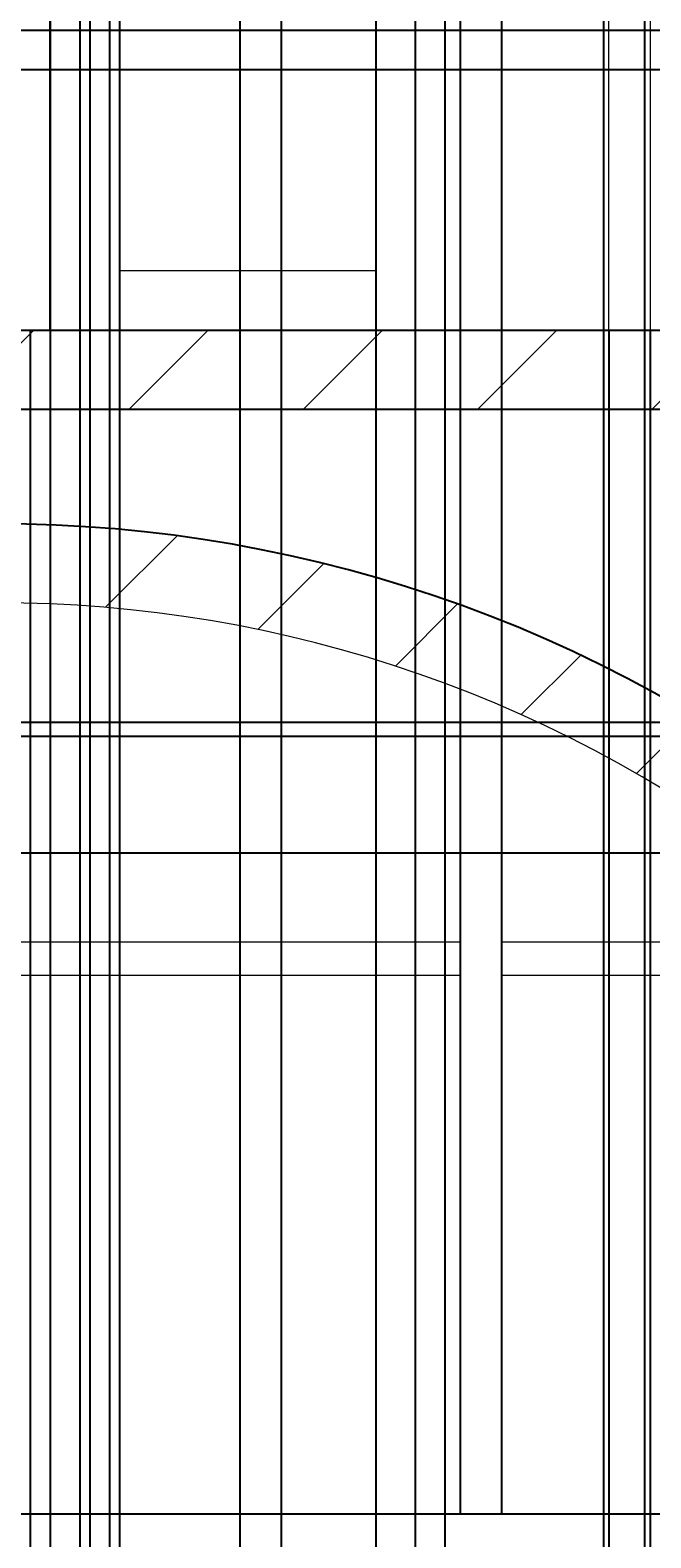
# Model space of a CAD drawing. Units: inches. Extents: x -14 to 375, y -86 to 549.
# Tile 4 of 12: x 227 to 290, y 4 to 156. Entities that reach past the tile are written whole.
import ezdxf

# ---------------------------------------------------------------- set-up
doc = ezdxf.new("R2010")
doc.units = ezdxf.units.IN
doc.header["$MEASUREMENT"] = 0
for name, color, linetype, lineweight in [('A-ANNO-DIMS', 2, 'Continuous', 18), ('A-DOOR', 3, 'Continuous', 18), ('A-ELEV', 7, 'Continuous', 25), ('A-ELEV-PATT', 8, 'Continuous', 13), ('A-GLAZ', 4, 'Continuous', 18)]:
    doc.layers.add(name, color=color, linetype=linetype, lineweight=lineweight)
doc.styles.get("Standard").update_dxf_attribs({"font": 'arial.ttf'})
doc.dimstyles.get("Standard").update_dxf_attribs({"dimtxt": 0.18, "dimasz": 0.18, "dimexe": 0.18, "dimexo": 0.0625, "dimgap": 0.09, "dimtad": 0, "dimtih": 1, "dimtoh": 1, "dimdec": 4, "dimzin": 0, "dimdsep": 46, "dimtxsty": 'Standard', "dimcen": 0.09, "dimadec": 0, "dimazin": 0, "dimtfac": 1, "dimtdec": 4, "dimtofl": 0, "dimtmove": 0, "dimatfit": 3, "dimfxl": 1, "dimtolj": 1, "dimtzin": 0, "dimarcsym": 0})

# ---------------------------------------------------------------- blocks, each defined once
blk = doc.blocks.new('*U3')
blk.add_lwpolyline([(3.12, 0.01), (0.12, 0.01), (0.12, 84.01), (40.12, 84.01), (40.12, 0.01), (37.12, 0.01)])
for points in [[(37.12, 80.99), (37.12, 0.01), (3.12, 0.01), (3.12, 80.99)], [(33.12, 6.01), (33.12, 74.99), (7.12, 74.99), (7.12, 6.01)]]:
    blk.add_lwpolyline(points, close=True)
blk.add_circle((35.12, 42.01), 1)
blk = doc.blocks.new('*D28')
at = {"layer": 'A-ANNO-DIMS', "color": 0, "lineweight": -2, "transparency": 16777216}
for p, q in [((107.764387, 156.376775), (374.544714, 156.376775)), ((374.364714, 156.196775), (374.364714, 154.556775)), ((374.364714, 152.556775), (374.364714, 154.196775)), ((111.764387, 152.376775), (374.544714, 152.376775))]:
    blk.add_line(p, q, dxfattribs=at)
at = {"layer": 'A-ANNO-DIMS', "color": 0, "transparency": 16777216}
for points in [[(374.334714, 156.196775), (374.394714, 156.196775), (374.364714, 156.376775)], [(374.334714, 152.556775), (374.394714, 152.556775), (374.364714, 152.376775)]]:
    blk.add_solid(points, dxfattribs=at)
at = {"layer": 'Defpoints', "color": 0, "transparency": 16777216}
for p in [(107.701887, 156.376775), (374.364714, 156.376775), (111.701887, 152.376775)]:
    blk.add_point(p, dxfattribs=at)
at = {"layer": 'A-ANNO-DIMS', "color": 0, "transparency": 16777216, "insert": (374.364714, 154.376775), "char_height": 0.18, "attachment_point": 5}
blk.add_mtext('\\A1;4', dxfattribs=at)
blk = doc.blocks.new('*D29')
at = {"layer": 'A-ANNO-DIMS', "color": 0, "lineweight": -2, "transparency": 16777216}
for p, q in [((107.74, 193.48), (374.54, 193.48)), ((374.36, 193.3), (374.36, 175.11)), ((374.36, 156.56), (374.36, 174.75)), ((107.76, 156.38), (374.54, 156.38))]:
    blk.add_line(p, q, dxfattribs=at)
at = {"layer": 'A-ANNO-DIMS', "color": 0, "transparency": 16777216}
for points in [[(374.33, 193.3), (374.39, 193.3), (374.36, 193.48)], [(374.33, 156.56), (374.39, 156.56), (374.36, 156.38)]]:
    blk.add_solid(points, dxfattribs=at)
at = {"layer": 'Defpoints', "color": 0, "transparency": 16777216}
for p in [(107.68, 193.48), (374.36, 193.48), (107.7, 156.38)]:
    blk.add_point(p, dxfattribs=at)
at = {"layer": 'A-ANNO-DIMS', "color": 0, "transparency": 16777216, "insert": (374.36, 174.93), "char_height": 0.18, "attachment_point": 5}
blk.add_mtext('\\A1;37.106', dxfattribs=at)
blk = doc.blocks.new('*D43')
at = {"layer": 'A-ANNO-DIMS', "color": 0, "lineweight": -2, "transparency": 16777216}
for p, q in [((142.23, 270.64), (142.23, -64.39)), ((305.63, 270.64), (305.63, -64.39)), ((142.41, -64.21), (223.55, -64.21)), ((305.45, -64.21), (224.32, -64.21))]:
    blk.add_line(p, q, dxfattribs=at)
at = {"layer": 'A-ANNO-DIMS', "color": 0, "transparency": 16777216}
for points in [[(142.41, -64.18), (142.41, -64.24), (142.23, -64.21)], [(305.45, -64.18), (305.45, -64.24), (305.63, -64.21)]]:
    blk.add_solid(points, dxfattribs=at)
at = {"layer": 'Defpoints', "color": 0, "transparency": 16777216}
for p in [(142.23, 270.71), (305.63, 270.71), (305.63, -64.21)]:
    blk.add_point(p, dxfattribs=at)
at = {"layer": 'A-ANNO-DIMS', "color": 0, "transparency": 16777216, "insert": (223.93, -64.21), "char_height": 0.18, "attachment_point": 5}
blk.add_mtext('\\A1;163.4', dxfattribs=at)
blk = doc.blocks.new('*D49')
at = {"layer": 'A-ANNO-DIMS', "color": 0, "lineweight": -2, "transparency": 16777216}
for p, q in [((215.95, 306.64), (215.95, -64.39)), ((248.64, 306.64), (248.64, -64.39)), ((216.13, -64.21), (231.9, -64.21)), ((248.46, -64.21), (232.69, -64.21))]:
    blk.add_line(p, q, dxfattribs=at)
at = {"layer": 'A-ANNO-DIMS', "color": 0, "transparency": 16777216}
for points in [[(216.13, -64.18), (216.13, -64.24), (215.95, -64.21)], [(248.46, -64.18), (248.46, -64.24), (248.64, -64.21)]]:
    blk.add_solid(points, dxfattribs=at)
at = {"layer": 'Defpoints', "color": 0, "transparency": 16777216}
for p in [(215.95, 306.71), (248.64, 306.71), (248.64, -64.21)]:
    blk.add_point(p, dxfattribs=at)
at = {"layer": 'A-ANNO-DIMS', "color": 0, "transparency": 16777216, "insert": (232.29, -64.21), "char_height": 0.18, "attachment_point": 5}
blk.add_mtext('\\A1;32.69', dxfattribs=at)
blk = doc.blocks.new('*D50')
at = {"layer": 'A-ANNO-DIMS', "color": 0, "lineweight": -2, "transparency": 16777216}
for p, q in [((248.64, 306.64), (248.64, -64.39)), ((252.81, 306.64), (252.81, -64.39)), ((248.82, -64.21), (250.39, -64.21)), ((252.63, -64.21), (251.05, -64.21))]:
    blk.add_line(p, q, dxfattribs=at)
at = {"layer": 'A-ANNO-DIMS', "color": 0, "transparency": 16777216}
for points in [[(248.82, -64.18), (248.82, -64.24), (248.64, -64.21)], [(252.63, -64.18), (252.63, -64.24), (252.81, -64.21)]]:
    blk.add_solid(points, dxfattribs=at)
at = {"layer": 'Defpoints', "color": 0, "transparency": 16777216}
for p in [(248.64, 306.71), (252.81, 306.71), (252.81, -64.21)]:
    blk.add_point(p, dxfattribs=at)
at = {"layer": 'A-ANNO-DIMS', "color": 0, "transparency": 16777216, "insert": (250.72, -64.21), "char_height": 0.18, "attachment_point": 5}
blk.add_mtext('\\A1;4.17', dxfattribs=at)
blk = doc.blocks.new('*D51')
at = {"layer": 'A-ANNO-DIMS', "color": 0, "lineweight": -2, "transparency": 16777216}
for p, q in [((252.81, 306.64), (252.81, -64.39)), ((285.5, 306.64), (285.5, -64.39)), ((252.99, -64.21), (268.76, -64.21)), ((285.32, -64.21), (269.54, -64.21))]:
    blk.add_line(p, q, dxfattribs=at)
at = {"layer": 'A-ANNO-DIMS', "color": 0, "transparency": 16777216}
for points in [[(252.99, -64.18), (252.99, -64.24), (252.81, -64.21)], [(285.32, -64.18), (285.32, -64.24), (285.5, -64.21)]]:
    blk.add_solid(points, dxfattribs=at)
at = {"layer": 'Defpoints', "color": 0, "transparency": 16777216}
for p in [(252.81, 306.71), (285.5, 306.71), (285.5, -64.21)]:
    blk.add_point(p, dxfattribs=at)
at = {"layer": 'A-ANNO-DIMS', "color": 0, "transparency": 16777216, "insert": (269.15, -64.21), "char_height": 0.18, "attachment_point": 5}
blk.add_mtext('\\A1;32.69', dxfattribs=at)
blk = doc.blocks.new('*D52')
at = {"layer": 'A-ANNO-DIMS', "color": 0, "lineweight": -2, "transparency": 16777216}
for p, q in [((285.5, 306.64), (285.5, -64.39)), ((289.66, 306.64), (289.66, -64.39)), ((285.68, -64.21), (287.25, -64.21)), ((289.48, -64.21), (287.91, -64.21))]:
    blk.add_line(p, q, dxfattribs=at)
at = {"layer": 'A-ANNO-DIMS', "color": 0, "transparency": 16777216}
for points in [[(285.68, -64.18), (285.68, -64.24), (285.5, -64.21)], [(289.48, -64.18), (289.48, -64.24), (289.66, -64.21)]]:
    blk.add_solid(points, dxfattribs=at)
at = {"layer": 'Defpoints', "color": 0, "transparency": 16777216}
for p in [(285.5, 306.71), (289.66, 306.71), (289.66, -64.21)]:
    blk.add_point(p, dxfattribs=at)
at = {"layer": 'A-ANNO-DIMS', "color": 0, "transparency": 16777216, "insert": (287.58, -64.21), "char_height": 0.18, "attachment_point": 5}
blk.add_mtext('\\A1;4.17', dxfattribs=at)
blk = doc.blocks.new('*D57')
at = {"layer": 'A-ANNO-DIMS', "color": 0, "lineweight": -2, "transparency": 16777216}
for p, q in [((229.41, 340.38), (229.41, -64.39)), ((232.41, 340.38), (232.41, -64.39)), ((229.59, -64.21), (230.76, -64.21)), ((232.23, -64.21), (231.06, -64.21))]:
    blk.add_line(p, q, dxfattribs=at)
at = {"layer": 'A-ANNO-DIMS', "color": 0, "transparency": 16777216}
for points in [[(229.59, -64.18), (229.59, -64.24), (229.41, -64.21)], [(232.23, -64.18), (232.23, -64.24), (232.41, -64.21)]]:
    blk.add_solid(points, dxfattribs=at)
at = {"layer": 'Defpoints', "color": 0, "transparency": 16777216}
for p in [(229.41, 340.44), (232.41, 340.44), (232.41, -64.21)]:
    blk.add_point(p, dxfattribs=at)
at = {"layer": 'A-ANNO-DIMS', "color": 0, "transparency": 16777216, "insert": (230.91, -64.21), "char_height": 0.18, "attachment_point": 5}
blk.add_mtext('\\A1;3', dxfattribs=at)
blk = doc.blocks.new('*D58')
at = {"layer": 'A-ANNO-DIMS', "color": 0, "lineweight": -2, "transparency": 16777216}
for p, q in [((232.41, 340.38), (232.41, -64.39)), ((236.41, 340.38), (236.41, -64.39)), ((232.59, -64.21), (234.26, -64.21)), ((236.23, -64.21), (234.56, -64.21))]:
    blk.add_line(p, q, dxfattribs=at)
at = {"layer": 'A-ANNO-DIMS', "color": 0, "transparency": 16777216}
for points in [[(232.59, -64.18), (232.59, -64.24), (232.41, -64.21)], [(236.23, -64.18), (236.23, -64.24), (236.41, -64.21)]]:
    blk.add_solid(points, dxfattribs=at)
at = {"layer": 'Defpoints', "color": 0, "transparency": 16777216}
for p in [(232.41, 340.44), (236.41, 340.44), (236.41, -64.21)]:
    blk.add_point(p, dxfattribs=at)
at = {"layer": 'A-ANNO-DIMS', "color": 0, "transparency": 16777216, "insert": (234.41, -64.21), "char_height": 0.18, "attachment_point": 5}
blk.add_mtext('\\A1;4', dxfattribs=at)
blk = doc.blocks.new('*D59')
at = {"layer": 'A-ANNO-DIMS', "color": 0, "lineweight": -2, "transparency": 16777216}
for p, q in [((236.41, 340.38), (236.41, -64.39)), ((262.41, 340.38), (262.41, -64.39)), ((236.59, -64.21), (249.19, -64.21)), ((262.23, -64.21), (249.63, -64.21))]:
    blk.add_line(p, q, dxfattribs=at)
at = {"layer": 'A-ANNO-DIMS', "color": 0, "transparency": 16777216}
for points in [[(236.59, -64.18), (236.59, -64.24), (236.41, -64.21)], [(262.23, -64.18), (262.23, -64.24), (262.41, -64.21)]]:
    blk.add_solid(points, dxfattribs=at)
at = {"layer": 'Defpoints', "color": 0, "transparency": 16777216}
for p in [(236.41, 340.44), (262.41, 340.44), (262.41, -64.21)]:
    blk.add_point(p, dxfattribs=at)
at = {"layer": 'A-ANNO-DIMS', "color": 0, "transparency": 16777216, "insert": (249.41, -64.21), "char_height": 0.18, "attachment_point": 5}
blk.add_mtext('\\A1;26', dxfattribs=at)
blk = doc.blocks.new('*D60')
at = {"layer": 'A-ANNO-DIMS', "color": 0, "lineweight": -2, "transparency": 16777216}
for p, q in [((262.41, 340.38), (262.41, -64.39)), ((266.41, 340.38), (266.41, -64.39)), ((262.59, -64.21), (264.26, -64.21)), ((266.23, -64.21), (264.56, -64.21))]:
    blk.add_line(p, q, dxfattribs=at)
at = {"layer": 'A-ANNO-DIMS', "color": 0, "transparency": 16777216}
for points in [[(262.59, -64.18), (262.59, -64.24), (262.41, -64.21)], [(266.23, -64.18), (266.23, -64.24), (266.41, -64.21)]]:
    blk.add_solid(points, dxfattribs=at)
at = {"layer": 'Defpoints', "color": 0, "transparency": 16777216}
for p in [(262.41, 340.44), (266.41, 340.44), (266.41, -64.21)]:
    blk.add_point(p, dxfattribs=at)
at = {"layer": 'A-ANNO-DIMS', "color": 0, "transparency": 16777216, "insert": (264.41, -64.21), "char_height": 0.18, "attachment_point": 5}
blk.add_mtext('\\A1;4', dxfattribs=at)
blk = doc.blocks.new('*D61')
at = {"layer": 'A-ANNO-DIMS', "color": 0, "lineweight": -2, "transparency": 16777216}
for p, q in [((266.41, 340.38), (266.41, -64.39)), ((269.41, 340.38), (269.41, -64.39)), ((266.59, -64.21), (267.76, -64.21)), ((269.23, -64.21), (268.06, -64.21))]:
    blk.add_line(p, q, dxfattribs=at)
at = {"layer": 'A-ANNO-DIMS', "color": 0, "transparency": 16777216}
for points in [[(266.59, -64.18), (266.59, -64.24), (266.41, -64.21)], [(269.23, -64.18), (269.23, -64.24), (269.41, -64.21)]]:
    blk.add_solid(points, dxfattribs=at)
at = {"layer": 'Defpoints', "color": 0, "transparency": 16777216}
for p in [(266.41, 340.44), (269.41, 340.44), (269.41, -64.21)]:
    blk.add_point(p, dxfattribs=at)
at = {"layer": 'A-ANNO-DIMS', "color": 0, "transparency": 16777216, "insert": (267.91, -64.21), "char_height": 0.18, "attachment_point": 5}
blk.add_mtext('\\A1;3', dxfattribs=at)
blk = doc.blocks.new('*D71')
at = {"layer": 'A-ANNO-DIMS', "color": 0, "lineweight": -2, "transparency": 16777216}
for p, q in [((233.41, 167.91), (233.41, -64.39)), ((235.41, 167.91), (235.41, -64.39)), ((233.59, -64.21), (234.26, -64.21)), ((235.23, -64.21), (234.56, -64.21))]:
    blk.add_line(p, q, dxfattribs=at)
at = {"layer": 'A-ANNO-DIMS', "color": 0, "transparency": 16777216}
for points in [[(233.59, -64.18), (233.59, -64.24), (233.41, -64.21)], [(235.23, -64.18), (235.23, -64.24), (235.41, -64.21)]]:
    blk.add_solid(points, dxfattribs=at)
at = {"layer": 'Defpoints', "color": 0, "transparency": 16777216}
for p in [(233.41, 167.97), (235.41, 167.97), (235.41, -64.21)]:
    blk.add_point(p, dxfattribs=at)
at = {"layer": 'A-ANNO-DIMS', "color": 0, "transparency": 16777216, "insert": (234.41, -64.21), "char_height": 0.18, "attachment_point": 5}
blk.add_mtext('\\A1;2', dxfattribs=at)
blk = doc.blocks.new('*D72')
at = {"layer": 'A-ANNO-DIMS', "color": 0, "lineweight": -2, "transparency": 16777216}
for p, q in [((229.41, 126.03), (229.41, 515.24)), ((233.41, 168.03), (233.41, 515.24)), ((229.59, 515.06), (231.26, 515.06)), ((233.23, 515.06), (231.56, 515.06))]:
    blk.add_line(p, q, dxfattribs=at)
at = {"layer": 'A-ANNO-DIMS', "color": 0, "transparency": 16777216}
for points in [[(229.59, 515.09), (229.59, 515.03), (229.41, 515.06)], [(233.23, 515.09), (233.23, 515.03), (233.41, 515.06)]]:
    blk.add_solid(points, dxfattribs=at)
at = {"layer": 'Defpoints', "color": 0, "transparency": 16777216}
for p in [(233.41, 515.06), (233.41, 167.97), (229.41, 125.97)]:
    blk.add_point(p, dxfattribs=at)
at = {"layer": 'A-ANNO-DIMS', "color": 0, "transparency": 16777216, "insert": (231.41, 515.06), "char_height": 0.18, "attachment_point": 5}
blk.add_mtext('\\A1;4', dxfattribs=at)
blk = doc.blocks.new('*D73')
at = {"layer": 'A-ANNO-DIMS', "color": 0, "lineweight": -2, "transparency": 16777216}
for p, q in [((234.47, 166.97), (374.54, 166.97)), ((374.36, 166.79), (374.36, 146.65)), ((374.36, 126.15), (374.36, 146.29)), ((269.47, 125.97), (374.54, 125.97))]:
    blk.add_line(p, q, dxfattribs=at)
at = {"layer": 'A-ANNO-DIMS', "color": 0, "transparency": 16777216}
for points in [[(374.33, 166.79), (374.39, 166.79), (374.36, 166.97)], [(374.33, 126.15), (374.39, 126.15), (374.36, 125.97)]]:
    blk.add_solid(points, dxfattribs=at)
at = {"layer": 'Defpoints', "color": 0, "transparency": 16777216}
for p in [(234.41, 166.97), (374.36, 166.97), (269.41, 125.97)]:
    blk.add_point(p, dxfattribs=at)
at = {"layer": 'A-ANNO-DIMS', "color": 0, "transparency": 16777216, "insert": (374.36, 146.47), "char_height": 0.18, "attachment_point": 5}
blk.add_mtext('\\A1;41', dxfattribs=at)
blk = doc.blocks.new('*D78')
at = {"layer": 'A-ANNO-DIMS', "color": 0, "lineweight": -2, "transparency": 16777216}
for p, q in [((187.37, 125.91), (187.37, -64.39)), ((227.37, 125.91), (227.37, -64.39)), ((187.55, -64.21), (207.14, -64.21)), ((227.19, -64.21), (207.59, -64.21))]:
    blk.add_line(p, q, dxfattribs=at)
at = {"layer": 'A-ANNO-DIMS', "color": 0, "transparency": 16777216}
for points in [[(187.55, -64.18), (187.55, -64.24), (187.37, -64.21)], [(227.19, -64.18), (227.19, -64.24), (227.37, -64.21)]]:
    blk.add_solid(points, dxfattribs=at)
at = {"layer": 'Defpoints', "color": 0, "transparency": 16777216}
for p in [(187.37, 125.97), (227.37, 125.97), (227.37, -64.21)]:
    blk.add_point(p, dxfattribs=at)
at = {"layer": 'A-ANNO-DIMS', "color": 0, "transparency": 16777216, "insert": (207.37, -64.21), "char_height": 0.18, "attachment_point": 5}
blk.add_mtext('\\A1;40', dxfattribs=at)
blk = doc.blocks.new('*D79')
at = {"layer": 'A-ANNO-DIMS', "color": 0, "lineweight": -2, "transparency": 16777216}
for p, q in [((227.37, 125.91), (227.37, -64.39)), ((229.41, 125.91), (229.41, -64.39)), ((227.55, -64.21), (228.06, -64.21)), ((229.23, -64.21), (228.71, -64.21))]:
    blk.add_line(p, q, dxfattribs=at)
at = {"layer": 'A-ANNO-DIMS', "color": 0, "transparency": 16777216}
for points in [[(227.55, -64.18), (227.55, -64.24), (227.37, -64.21)], [(229.23, -64.18), (229.23, -64.24), (229.41, -64.21)]]:
    blk.add_solid(points, dxfattribs=at)
at = {"layer": 'Defpoints', "color": 0, "transparency": 16777216}
for p in [(227.37, 125.97), (229.41, 125.97), (229.41, -64.21)]:
    blk.add_point(p, dxfattribs=at)
at = {"layer": 'A-ANNO-DIMS', "color": 0, "transparency": 16777216, "insert": (228.39, -64.21), "char_height": 0.18, "attachment_point": 5}
blk.add_mtext('\\A1;2.04', dxfattribs=at)
blk = doc.blocks.new('*D80')
at = {"layer": 'A-ANNO-DIMS', "color": 0, "lineweight": -2, "transparency": 16777216}
for p, q in [((229.41, 125.91), (229.41, -64.39)), ((269.41, 125.91), (269.41, -64.39)), ((229.59, -64.21), (249.19, -64.21)), ((269.23, -64.21), (249.63, -64.21))]:
    blk.add_line(p, q, dxfattribs=at)
at = {"layer": 'A-ANNO-DIMS', "color": 0, "transparency": 16777216}
for points in [[(229.59, -64.18), (229.59, -64.24), (229.41, -64.21)], [(269.23, -64.18), (269.23, -64.24), (269.41, -64.21)]]:
    blk.add_solid(points, dxfattribs=at)
at = {"layer": 'Defpoints', "color": 0, "transparency": 16777216}
for p in [(229.41, 125.97), (269.41, 125.97), (269.41, -64.21)]:
    blk.add_point(p, dxfattribs=at)
at = {"layer": 'A-ANNO-DIMS', "color": 0, "transparency": 16777216, "insert": (249.41, -64.21), "char_height": 0.18, "attachment_point": 5}
blk.add_mtext('\\A1;40', dxfattribs=at)
blk = doc.blocks.new('*D81')
at = {"layer": 'A-ANNO-DIMS', "color": 0, "lineweight": -2, "transparency": 16777216}
for p, q in [((269.41, 125.91), (269.41, -64.39)), ((286.05, 125.9), (286.05, -64.39)), ((269.59, -64.21), (277.34, -64.21)), ((285.87, -64.21), (278.11, -64.21))]:
    blk.add_line(p, q, dxfattribs=at)
at = {"layer": 'A-ANNO-DIMS', "color": 0, "transparency": 16777216}
for points in [[(269.59, -64.18), (269.59, -64.24), (269.41, -64.21)], [(285.87, -64.18), (285.87, -64.24), (286.05, -64.21)]]:
    blk.add_solid(points, dxfattribs=at)
at = {"layer": 'Defpoints', "color": 0, "transparency": 16777216}
for p in [(269.41, 125.97), (286.05, 125.96), (286.05, -64.21)]:
    blk.add_point(p, dxfattribs=at)
at = {"layer": 'A-ANNO-DIMS', "color": 0, "transparency": 16777216, "insert": (277.73, -64.21), "char_height": 0.18, "attachment_point": 5}
blk.add_mtext('\\A1;16.64', dxfattribs=at)
blk = doc.blocks.new('*D82')
at = {"layer": 'A-ANNO-DIMS', "color": 0, "lineweight": -2, "transparency": 16777216}
for p, q in [((286.05, 125.9), (286.05, -64.39)), ((290.24, 125.9), (290.24, -64.39)), ((286.23, -64.21), (287.75, -64.21)), ((290.06, -64.21), (288.54, -64.21))]:
    blk.add_line(p, q, dxfattribs=at)
at = {"layer": 'A-ANNO-DIMS', "color": 0, "transparency": 16777216}
for points in [[(286.23, -64.18), (286.23, -64.24), (286.05, -64.21)], [(290.06, -64.18), (290.06, -64.24), (290.24, -64.21)]]:
    blk.add_solid(points, dxfattribs=at)
at = {"layer": 'Defpoints', "color": 0, "transparency": 16777216}
for p in [(286.05, 125.96), (290.24, 125.96), (290.24, -64.21)]:
    blk.add_point(p, dxfattribs=at)
at = {"layer": 'A-ANNO-DIMS', "color": 0, "transparency": 16777216, "insert": (288.14, -64.21), "char_height": 0.18, "attachment_point": 5}
blk.add_mtext('\\A1;4.186', dxfattribs=at)
blk = doc.blocks.new('*D83')
at = {"layer": 'A-ANNO-DIMS', "color": 0, "lineweight": -2, "transparency": 16777216}
for p, q in [((290.24, 125.9), (290.24, -64.39)), ((305.77, 125.9), (305.77, -64.39)), ((290.42, -64.21), (297.55, -64.21)), ((305.59, -64.21), (298.46, -64.21))]:
    blk.add_line(p, q, dxfattribs=at)
at = {"layer": 'A-ANNO-DIMS', "color": 0, "transparency": 16777216}
for points in [[(290.42, -64.18), (290.42, -64.24), (290.24, -64.21)], [(305.59, -64.18), (305.59, -64.24), (305.77, -64.21)]]:
    blk.add_solid(points, dxfattribs=at)
at = {"layer": 'Defpoints', "color": 0, "transparency": 16777216}
for p in [(290.24, 125.96), (305.77, 125.96), (305.77, -64.21)]:
    blk.add_point(p, dxfattribs=at)
at = {"layer": 'A-ANNO-DIMS', "color": 0, "transparency": 16777216, "insert": (298, -64.21), "char_height": 0.18, "attachment_point": 5}
blk.add_mtext('\\A1;15.534', dxfattribs=at)
blk = doc.blocks.new('*D104')
at = {"layer": 'A-ANNO-DIMS', "color": 0, "lineweight": -2, "transparency": 16777216}
for p, q in [((190.15, 6.02), (190.15, 515.24)), ((271, 6.02), (271, 515.24)), ((190.33, 515.06), (230.18, 515.06)), ((270.82, 515.06), (230.97, 515.06))]:
    blk.add_line(p, q, dxfattribs=at)
at = {"layer": 'A-ANNO-DIMS', "color": 0, "transparency": 16777216}
for points in [[(190.33, 515.09), (190.33, 515.03), (190.15, 515.06)], [(270.82, 515.09), (270.82, 515.03), (271, 515.06)]]:
    blk.add_solid(points, dxfattribs=at)
at = {"layer": 'Defpoints', "color": 0, "transparency": 16777216}
for p in [(271, 515.06), (190.15, 5.96), (271, 5.96)]:
    blk.add_point(p, dxfattribs=at)
at = {"layer": 'A-ANNO-DIMS', "color": 0, "transparency": 16777216, "insert": (230.57, 515.06), "char_height": 0.18, "attachment_point": 5}
blk.add_mtext('\\A1;80.85', dxfattribs=at)
blk = doc.blocks.new('*D105')
at = {"layer": 'A-ANNO-DIMS', "color": 0, "lineweight": -2, "transparency": 16777216}
for p, q in [((271, 6.02), (271, 515.24)), ((275.19, 6.02), (275.19, 515.24)), ((271.18, 515.06), (272.69, 515.06)), ((275.01, 515.06), (273.49, 515.06))]:
    blk.add_line(p, q, dxfattribs=at)
at = {"layer": 'A-ANNO-DIMS', "color": 0, "transparency": 16777216}
for points in [[(271.18, 515.09), (271.18, 515.03), (271, 515.06)], [(275.01, 515.09), (275.01, 515.03), (275.19, 515.06)]]:
    blk.add_solid(points, dxfattribs=at)
at = {"layer": 'Defpoints', "color": 0, "transparency": 16777216}
for p in [(275.19, 515.06), (271, 5.96), (275.19, 5.96)]:
    blk.add_point(p, dxfattribs=at)
at = {"layer": 'A-ANNO-DIMS', "color": 0, "transparency": 16777216, "insert": (273.09, 515.06), "char_height": 0.18, "attachment_point": 5}
blk.add_mtext('\\A1;4.186', dxfattribs=at)
blk = doc.blocks.new('*D106')
at = {"layer": 'A-ANNO-DIMS', "color": 0, "lineweight": -2, "transparency": 16777216}
for p, q in [((275.19, 6.02), (275.19, 515.24)), ((305.77, 6.02), (305.77, 515.24)), ((275.37, 515.06), (290.01, 515.06)), ((305.59, 515.06), (290.94, 515.06))]:
    blk.add_line(p, q, dxfattribs=at)
at = {"layer": 'A-ANNO-DIMS', "color": 0, "transparency": 16777216}
for points in [[(275.37, 515.09), (275.37, 515.03), (275.19, 515.06)], [(305.59, 515.09), (305.59, 515.03), (305.77, 515.06)]]:
    blk.add_solid(points, dxfattribs=at)
at = {"layer": 'Defpoints', "color": 0, "transparency": 16777216}
for p in [(305.77, 515.06), (275.19, 5.96), (305.77, 5.96)]:
    blk.add_point(p, dxfattribs=at)
at = {"layer": 'A-ANNO-DIMS', "color": 0, "transparency": 16777216, "insert": (290.48, 515.06), "char_height": 0.18, "attachment_point": 5}
blk.add_mtext('\\A1;30.585', dxfattribs=at)
blk = doc.blocks.new('*D128')
at = {"layer": 'A-ANNO-DIMS', "color": 0, "lineweight": -2, "transparency": 16777216}
for p, q in [((96.79, 84.82), (374.54, 84.82)), ((374.36, 84.64), (374.36, 79.07)), ((374.36, 73.15), (374.36, 78.71)), ((111.56, 72.97), (374.54, 72.97))]:
    blk.add_line(p, q, dxfattribs=at)
at = {"layer": 'A-ANNO-DIMS', "color": 0, "transparency": 16777216}
for points in [[(374.33, 84.64), (374.39, 84.64), (374.36, 84.82)], [(374.33, 73.15), (374.39, 73.15), (374.36, 72.97)]]:
    blk.add_solid(points, dxfattribs=at)
at = {"layer": 'Defpoints', "color": 0, "transparency": 16777216}
for p in [(96.73, 84.82), (374.36, 84.82), (111.5, 72.97)]:
    blk.add_point(p, dxfattribs=at)
at = {"layer": 'A-ANNO-DIMS', "color": 0, "transparency": 16777216, "insert": (374.36, 78.89), "char_height": 0.18, "attachment_point": 5}
blk.add_mtext('\\A1;11.849', dxfattribs=at)
blk = doc.blocks.new('*D129')
at = {"layer": 'A-ANNO-DIMS', "color": 0, "lineweight": -2, "transparency": 16777216}
for p, q in [((96.79, 86.23), (374.54, 86.23)), ((374.36, 86.05), (374.36, 85.7)), ((96.79, 84.82), (374.54, 84.82)), ((374.36, 85), (374.36, 85.34))]:
    blk.add_line(p, q, dxfattribs=at)
at = {"layer": 'A-ANNO-DIMS', "color": 0, "transparency": 16777216}
for points in [[(374.33, 86.05), (374.39, 86.05), (374.36, 86.23)], [(374.33, 85), (374.39, 85), (374.36, 84.82)]]:
    blk.add_solid(points, dxfattribs=at)
at = {"layer": 'Defpoints', "color": 0, "transparency": 16777216}
for p in [(96.73, 86.23), (374.36, 86.23), (96.73, 84.82)]:
    blk.add_point(p, dxfattribs=at)
at = {"layer": 'A-ANNO-DIMS', "color": 0, "transparency": 16777216, "insert": (374.36, 85.52), "char_height": 0.18, "attachment_point": 5}
blk.add_mtext('\\A1;1.409', dxfattribs=at)

msp = doc.modelspace()

# ---------------------------------------------------------------- hatches: boundary and pattern name
at = {"layer": 'A-ELEV-PATT'}
h = msp.add_hatch(dxfattribs=at)
h.set_pattern_fill('ANSI31', color=256, scale=100)
h.set_pattern_definition([(45, (-168.406, -22.703), (-8.83883, 8.83883), [])])
h.paths.add_polyline_path([(313.6281, 262.7071), (313.6281, 357.9589), (313.7701, 357.9589), (313.7701, 433.1717, 0.36940998), (134.2334, 433.1717), (134.2334, 365.9589), (134.2334, 262.7071)])
h.paths.add_polyline_path([(142.2334, 270.7071), (142.2334, 365.9589), (142.2334, 429.4208, -0.35358711), (305.7701, 429.4208), (305.7701, 365.9589), (305.6281, 365.9589), (305.6281, 270.7071)], flags=16)
h.paths.add_polyline_path([(134.2334, 187.8466), (134.2334, 117.9589), (313.7701, 117.9589), (313.7701, 187.8466, 0.62486768)])
h.paths.add_polyline_path([(305.7701, 185.9589), (305.7701, 125.9589), (142.2334, 125.9589), (142.2334, 185.9589, -0.61125102)], flags=16)
h.paths.add_polyline_path([(134.2334, 73.1717), (134.2334, 5.9589), (142.2334, 5.9589), (142.2334, 69.4208, -0.35358711), (305.7701, 69.4208), (305.7701, 5.9589), (313.7701, 5.9589), (313.7701, 73.1717, 0.36940998)])

# ---------------------------------------------------------------- linework, layer by layer
at = {"layer": 'A-ELEV'}
msp.add_line((15.4018, 5.9589), (345.2647, 5.9589), dxfattribs=at)
for points in [[(134.2334, 187.8466), (134.2334, 117.9589), (313.7701, 117.9589), (313.7701, 187.8466, 0.62486768)], [(142.2334, 185.9589), (142.2334, 125.9589), (305.7701, 125.9589), (305.7701, 185.9589, 0.61125102)]]:
    msp.add_lwpolyline(points, format="xyb", close=True, dxfattribs=at)
msp.add_lwpolyline([(313.7701, 5.9589), (313.7701, 73.1717, 0.36940998), (134.2334, 73.1717), (134.2334, 5.9589)], format="xyb", dxfattribs=at)
for points in [[(15.4018, 5.9589), (345.2647, 5.9589), (345.2647, -35.1115), (15.4018, -35.1115)], [(152.9633, 5.9589), (297.193, 5.9589), (297.193, -7.7312), (152.9633, -7.7312)]]:
    msp.add_lwpolyline(points, close=True, dxfattribs=at)
at = {"layer": 'A-GLAZ'}
for points in [[(290.2356, 176.9318), (290.2356, 125.9589), (286.0499, 125.9589), (286.0499, 211.8227)], [(270.9993, 63.9218), (270.9993, 89.5464)], [(275.185, 87.8404), (275.185, 63.9218)], [(270.9993, 63.9218), (190.148, 63.9218)], [(275.185, 60.5886), (305.7701, 60.5886), (305.7701, 63.9218), (275.185, 63.9218)], [(190.148, 60.5886), (270.9993, 60.5886)], [(275.185, 60.5886), (275.185, 5.9589), (270.9993, 5.9589), (270.9993, 60.5886)]]:
    msp.add_lwpolyline(points, dxfattribs=at)
msp.add_lwpolyline([(305.7701, 5.9589), (305.7701, 69.4208, 0.35358711), (142.2334, 69.4208), (142.2334, 5.9589)], format="xyb", dxfattribs=at)

# ---------------------------------------------------------------- block references
at = {"layer": 'A-DOOR', "xscale": -1}
msp.add_blockref('*U3', (269.5328, 125.9589), dxfattribs=at)

# ---------------------------------------------------------------- dimensions: what is measured, and where the dimension line sits
at = {"layer": 'A-ANNO-DIMS'}
for base, p1, p2, override, picture, middle in [((270.9993, 515.0589), (190.148, 5.9589), (270.9993, 5.9589), {"dimdec": 2, "dimlfac": 1, "dimrnd": 0, "dimzin": 0, "dimdsep": 46, "dimlunit": 2}, '*D104', (230.5736, 515.0589)), ((233.409, 515.0589), (229.409, 125.9717), (233.409, 167.9717), {"dimdec": 0, "dimlfac": 1, "dimrnd": 0, "dimzin": 0, "dimdsep": 46, "dimlunit": 2}, '*D72', (231.409, 515.0589)), ((275.185, 515.0589), (270.9993, 5.9589), (275.185, 5.9589), {"dimdec": 3, "dimlfac": 1, "dimrnd": 0, "dimzin": 0, "dimdsep": 46, "dimlunit": 2}, '*D105', (273.0921, 515.0589)), ((305.7701, 515.0589), (275.185, 5.9589), (305.7701, 5.9589), {"dimdec": 3, "dimlfac": 1, "dimrnd": 0, "dimzin": 0, "dimdsep": 46, "dimlunit": 2}, '*D106', (290.4775, 515.0589)), ((232.409, -64.2115), (229.409, 340.4421), (232.409, 340.4421), {"dimdec": 0, "dimlfac": 1, "dimrnd": 0, "dimzin": 0, "dimdsep": 46, "dimlunit": 2}, '*D57', (230.909, -64.2115)), ((236.409, -64.2115), (232.409, 340.4421), (236.409, 340.4421), {"dimdec": 0, "dimlfac": 1, "dimrnd": 0, "dimzin": 0, "dimdsep": 46, "dimlunit": 2}, '*D58', (234.409, -64.2115)), ((262.409, -64.2115), (236.409, 340.4421), (262.409, 340.4421), {"dimdec": 0, "dimlfac": 1, "dimrnd": 0, "dimzin": 0, "dimdsep": 46, "dimlunit": 2}, '*D59', (249.409, -64.2115)), ((266.409, -64.2115), (262.409, 340.4421), (266.409, 340.4421), {"dimdec": 0, "dimlfac": 1, "dimrnd": 0, "dimzin": 0, "dimdsep": 46, "dimlunit": 2}, '*D60', (264.409, -64.2115)), ((269.409, -64.2115), (266.409, 340.4421), (269.409, 340.4421), {"dimdec": 0, "dimlfac": 1, "dimrnd": 0, "dimzin": 0, "dimdsep": 46, "dimlunit": 2}, '*D61', (267.909, -64.2115)), ((248.639, -64.2115), (215.9481, 306.7071), (248.639, 306.7071), {"dimdec": 2, "dimlfac": 1, "dimrnd": 0, "dimzin": 0, "dimdsep": 46, "dimlunit": 2}, '*D49', (232.2936, -64.2115)), ((252.8055, -64.2115), (248.639, 306.7071), (252.8055, 306.7071), {"dimdec": 2, "dimlfac": 1, "dimrnd": 0, "dimzin": 0, "dimdsep": 46, "dimlunit": 2}, '*D50', (250.7222, -64.2115)), ((285.4964, -64.2115), (252.8055, 306.7071), (285.4964, 306.7071), {"dimdec": 2, "dimlfac": 1, "dimrnd": 0, "dimzin": 0, "dimdsep": 46, "dimlunit": 2}, '*D51', (269.1509, -64.2115)), ((289.6628, -64.2115), (285.4964, 306.7071), (289.6628, 306.7071), {"dimdec": 2, "dimlfac": 1, "dimrnd": 0, "dimzin": 0, "dimdsep": 46, "dimlunit": 2}, '*D52', (287.5796, -64.2115)), ((305.6281, -64.2115), (142.2334, 270.7071), (305.6281, 270.7071), {"dimdec": 1, "dimlfac": 1, "dimrnd": 0, "dimzin": 0, "dimdsep": 46, "dimlunit": 2}, '*D43', (223.9307, -64.2115)), ((235.409, -64.2115), (233.409, 167.9717), (235.409, 167.9717), {"dimdec": 0, "dimlfac": 1, "dimrnd": 0, "dimzin": 0, "dimdsep": 46, "dimlunit": 2}, '*D71', (234.409, -64.2115)), ((227.3657, -64.2115), (187.3657, 125.9717), (227.3657, 125.9717), {"dimdec": 0, "dimlfac": 1, "dimrnd": 0, "dimzin": 0, "dimdsep": 46, "dimlunit": 2}, '*D78', (207.3657, -64.2115)), ((229.409, -64.2115), (227.3657, 125.9717), (229.409, 125.9717), {"dimdec": 2, "dimlfac": 1, "dimrnd": 0, "dimzin": 0, "dimdsep": 46, "dimlunit": 2}, '*D79', (228.3874, -64.2115)), ((269.409, -64.2115), (229.409, 125.9717), (269.409, 125.9717), {"dimdec": 0, "dimlfac": 1, "dimrnd": 0, "dimzin": 0, "dimdsep": 46, "dimlunit": 2}, '*D80', (249.409, -64.2115)), ((286.0499, -64.2115), (269.409, 125.9717), (286.0499, 125.9589), {"dimdec": 2, "dimlfac": 1, "dimrnd": 0, "dimzin": 0, "dimdsep": 46, "dimlunit": 2}, '*D81', (277.7294, -64.2115)), ((290.2356, -64.2115), (286.0499, 125.9589), (290.2356, 125.9589), {"dimdec": 3, "dimlfac": 1, "dimrnd": 0, "dimzin": 0, "dimdsep": 46, "dimlunit": 2}, '*D82', (288.1427, -64.2115)), ((305.77006, -64.21154), (290.23562, 125.95892), (305.77006, 125.95892), {"dimdec": 3, "dimlfac": 1, "dimrnd": 0, "dimzin": 0, "dimdsep": 46, "dimlunit": 2}, '*D83', (298.00284, -64.21154))]:
    dim = msp.add_linear_dim(base=base, p1=p1, p2=p2, dimstyle='Standard', override=override, dxfattribs=at)
    dim.commit()
    dim.dimension.update_dxf_attribs({"geometry": picture, "text_midpoint": middle})
for base, p1, p2, override, picture, middle in [((374.3647, 193.4825), (107.7019, 156.3768), (107.6798, 193.4825), {"dimdec": 3, "dimlfac": 1, "dimrnd": 0, "dimzin": 0, "dimdsep": 46, "dimlunit": 2}, '*D29', (374.3647, 174.9296)), ((374.3647, 166.9717), (269.409, 125.9717), (234.409, 166.9717), {"dimdec": 0, "dimlfac": 1, "dimrnd": 0, "dimzin": 0, "dimdsep": 46, "dimlunit": 2}, '*D73', (374.3647, 146.4717)), ((374.3647, 156.3768), (111.7019, 152.3768), (107.7019, 156.3768), {"dimdec": 0, "dimlfac": 1, "dimrnd": 0, "dimzin": 0, "dimdsep": 46, "dimlunit": 2}, '*D28', (374.3647, 154.3768)), ((374.3647, 86.2255), (96.7255, 84.8165), (96.7255, 86.2255), {"dimdec": 3, "dimlfac": 1, "dimrnd": 0, "dimzin": 0, "dimdsep": 46, "dimlunit": 2}, '*D129', (374.3647, 85.521)), ((374.3647, 84.8165), (111.4987, 72.9679), (96.7255, 84.8165), {"dimdec": 3, "dimlfac": 1, "dimrnd": 0, "dimzin": 0, "dimdsep": 46, "dimlunit": 2}, '*D128', (374.3647, 78.8922))]:
    dim = msp.add_linear_dim(base=base, p1=p1, p2=p2, angle=90, dimstyle='Standard', override=override, dxfattribs=at)
    dim.commit()
    dim.dimension.update_dxf_attribs({"geometry": picture, "text_midpoint": middle})

doc.saveas('drawing.dxf')
